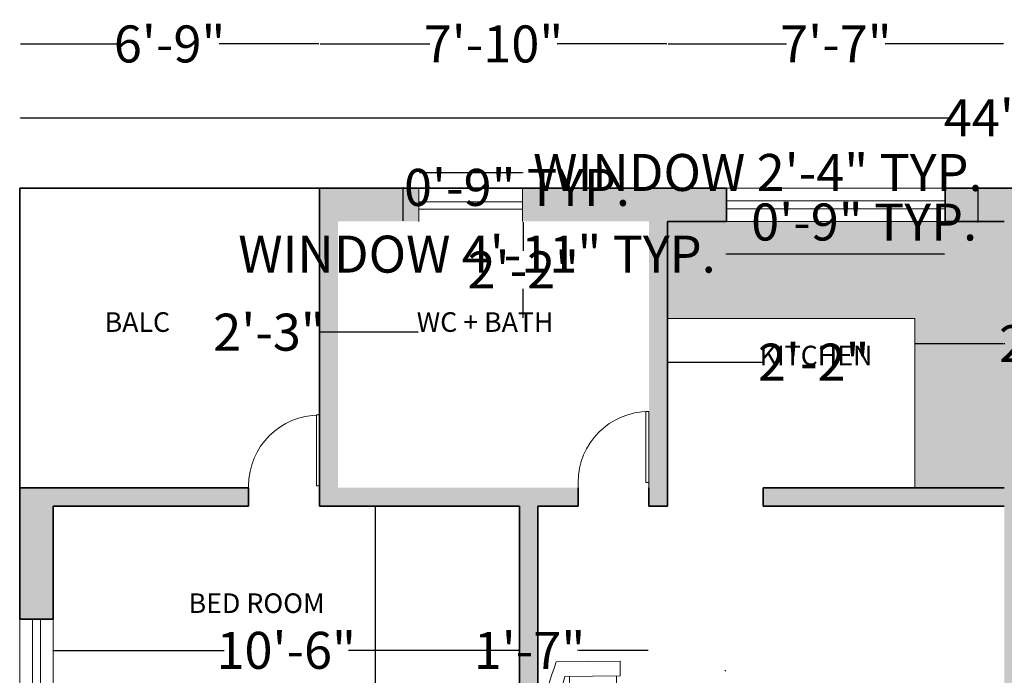
# Model space of a CAD drawing. Units: inches. Extents: x 1198 to 8596, y 144 to 930.
# Tile 4 of 5: x 1348 to 1614, y 753 to 930. Entities that reach past the tile are written whole.
import ezdxf

# ---------------------------------------------------------------- set-up
doc = ezdxf.new("R2010")
doc.units = ezdxf.units.IN
doc.header["$MEASUREMENT"] = 0
doc.layers.get('0').update_dxf_attribs({"color": 50})
for name, color, linetype, lineweight in [('A-ANNO-DIMS', 7, 'Continuous', 18), ('A-AREA-IDEN', 7, 'Continuous', 18), ('A-DOOR', 120, 'Continuous', 18), ('A-FLOR-FIXT', 8, 'Continuous', 18), ('A-FLOR-FIXT-PATT', 150, 'Continuous', 13), ('A-FURN', 11, 'Continuous', 18), ('A-WALL-PATT', 150, 'Continuous', 13), ('WALL', 7, 'Continuous', 35), ('WINDOW', 2, 'Continuous', 18)]:
    doc.layers.add(name, color=color, linetype=linetype, lineweight=lineweight)
doc.styles.get("Standard").update_dxf_attribs({"font": 'arial.ttf'})
doc.dimstyles.get("Standard").update_dxf_attribs({"dimtxt": 10, "dimasz": 0.18, "dimexe": 0.18, "dimexo": 0.0625, "dimgap": 0.09, "dimtad": 0, "dimtih": 1, "dimtoh": 1, "dimdec": 0, "dimzin": 0, "dimdsep": 46, "dimlunit": 3, "dimtxsty": 'Standard', "dimcen": 0.09, "dimse1": 1, "dimse2": 1, "dimadec": 0, "dimazin": 0, "dimtfac": 1, "dimtdec": 0, "dimtofl": 0, "dimtmove": 0, "dimatfit": 3, "dimfxl": 1, "dimtolj": 1, "dimtzin": 0, "dimarcsym": 0})

# ---------------------------------------------------------------- blocks, each defined once
blk = doc.blocks.new('WD_WIN4')
for p, q in [((-0.5, 0.5), (0.5, 0.5)), ((-0.5, 0.12), (0.5, 0.12)), ((-0.5, -0.12), (0.5, -0.12)), ((-0.5, -0.5), (0.5, -0.5))]:
    blk.add_line(p, q)
blk = doc.blocks.new('*U12')
for p, q in [((0, 0), (0, -6)), ((-40, 0), (-40, -6))]:
    blk.add_line(p, q)
blk.add_lwpolyline([(0, 0), (0, 40), (-1.75, 40), (-1.75, 0)], close=True)
blk.add_arc((0, 0), 40, 90, 180)
blk = doc.blocks.new('Sofa - Roundback 7 ft.')
for p, q in [((-12.00002, -32.4421), (-12.00003, -6.5971)), ((11.99997, -32.4421), (11.99998, -6.5971)), ((-36.000027, -34), (-36.000027, -11.4696)), ((35.99998, -34), (35.99998, -11.4696)), ((-35.999844, -13.3819), (35.9998, -13.3819)), ((-36.000027, -32.4421), (35.99998, -32.4421))]:
    blk.add_line(p, q)
for points in [[(-36.000027, -34), (-42.000027, -34), (-42.000027, -8)], [(41.99998, -8), (41.99998, -34), (35.99998, -34)]]:
    blk.add_lwpolyline(points)
for centre, radius, start, end in [((0, -114.25), 114.25, 68.43141, 111.5686), ((-0.00001, -127.1968), 121.1968, 72.72033, 107.2797)]:
    blk.add_arc(centre, radius, start, end)
blk = doc.blocks.new('*D15')
at = {"layer": 'A-ANNO-DIMS', "color": 0, "lineweight": -2, "transparency": 16777216}
for p, q in [((1348.07, 903.88), (1598.92, 903.88)), ((1884.71, 903.88), (1633.85, 903.88))]:
    blk.add_line(p, q, dxfattribs=at)
at = {"layer": 'A-ANNO-DIMS', "color": 0, "transparency": 16777216}
for points in [[(1348.07, 903.91), (1348.07, 903.85), (1347.89, 903.88)], [(1884.71, 903.91), (1884.71, 903.85), (1884.89, 903.88)]]:
    blk.add_solid(points, dxfattribs=at)
at = {"layer": 'Defpoints', "color": 0, "transparency": 16777216}
for p in [(1347.89, 903.88), (1347.89, 884.9), (1884.89, 884.9)]:
    blk.add_point(p, dxfattribs=at)
at = {"layer": 'A-ANNO-DIMS', "color": 0, "transparency": 16777216, "insert": (1616.39, 903.88), "char_height": 10, "attachment_point": 5}
blk.add_mtext('\\A1;44\'-9"', dxfattribs=at)
blk = doc.blocks.new('*D16')
at = {"layer": 'A-ANNO-DIMS', "color": 0, "lineweight": -2, "transparency": 16777216}
for p, q in [((1337.03, 884.72), (1337.03, 736.59)), ((1337.03, 578.08), (1337.03, 726.2))]:
    blk.add_line(p, q, dxfattribs=at)
at = {"layer": 'A-ANNO-DIMS', "color": 0, "transparency": 16777216}
for points in [[(1337, 884.72), (1337.06, 884.72), (1337.03, 884.9)], [(1337, 578.08), (1337.06, 578.08), (1337.03, 577.9)]]:
    blk.add_solid(points, dxfattribs=at)
at = {"layer": 'Defpoints', "color": 0, "transparency": 16777216}
for p in [(1347.89, 884.9), (1337.03, 577.9), (1347.89, 577.9)]:
    blk.add_point(p, dxfattribs=at)
at = {"layer": 'A-ANNO-DIMS', "color": 0, "transparency": 16777216, "insert": (1337.03, 731.4), "char_height": 10, "attachment_point": 5}
blk.add_mtext('\\A1;25\'-7"', dxfattribs=at)
blk = doc.blocks.new('*D17')
at = {"layer": 'A-ANNO-DIMS', "color": 0, "lineweight": -2, "transparency": 16777216}
for p, q in [((1288.75, 884.72), (1288.75, 551.09)), ((1288.75, 207.08), (1288.75, 540.7))]:
    blk.add_line(p, q, dxfattribs=at)
at = {"layer": 'A-ANNO-DIMS', "color": 0, "transparency": 16777216}
for points in [[(1288.72, 884.72), (1288.78, 884.72), (1288.75, 884.9)], [(1288.72, 207.08), (1288.78, 207.08), (1288.75, 206.9)]]:
    blk.add_solid(points, dxfattribs=at)
at = {"layer": 'Defpoints', "color": 0, "transparency": 16777216}
for p in [(1347.89, 884.9), (1288.75, 206.9), (1347.89, 206.9)]:
    blk.add_point(p, dxfattribs=at)
at = {"layer": 'A-ANNO-DIMS', "color": 0, "transparency": 16777216, "insert": (1288.75, 545.9), "char_height": 10, "attachment_point": 5}
blk.add_mtext('\\A1;56\'-6"', dxfattribs=at)
blk = doc.blocks.new('WIN-NARROW-28IN')
for p, q in [((0, 9), (0, 0)), ((28.06, 9), (28.06, 0)), ((0, 5.31), (28.06, 5.31)), ((0, 3.31), (28.06, 3.31))]:
    blk.add_line(p, q)
blk = doc.blocks.new('*D22')
at = {"layer": 'A-ANNO-DIMS', "color": 0, "lineweight": -2, "transparency": 16777216}
for p, q in [((1538.86, 867.04), (1538.68, 867.04)), ((1597.73, 867.04), (1539.04, 867.04))]:
    blk.add_line(p, q, dxfattribs=at)
at = {"layer": 'A-ANNO-DIMS', "color": 0, "transparency": 16777216}
for points in [[(1539.04, 867.07), (1539.04, 867.01), (1538.86, 867.04)], [(1597.73, 867.07), (1597.73, 867.01), (1597.91, 867.04)]]:
    blk.add_solid(points, dxfattribs=at)
at = {"layer": 'Defpoints', "color": 0, "transparency": 16777216}
for p in [(1538.86, 875.9), (1597.91, 875.9), (1538.86, 867.04)]:
    blk.add_point(p, dxfattribs=at)
at = {"layer": 'A-ANNO-DIMS', "color": 0, "transparency": 16777216, "insert": (1471.43, 867.04), "char_height": 10, "attachment_point": 5}
blk.add_mtext('\\A1;WINDOW 4\'-11" TYP.', dxfattribs=at)
blk = doc.blocks.new('*D23')
at = {"layer": 'A-ANNO-DIMS', "color": 0, "lineweight": -2, "transparency": 16777216}
for p, q in [((1606.77, 884.72), (1606.77, 876.08)), ((1606.77, 875.72), (1606.59, 875.72)), ((1606.77, 875.9), (1606.77, 875.72))]:
    blk.add_line(p, q, dxfattribs=at)
at = {"layer": 'A-ANNO-DIMS', "color": 0, "transparency": 16777216}
for points in [[(1606.74, 884.72), (1606.8, 884.72), (1606.77, 884.9)], [(1606.74, 876.08), (1606.8, 876.08), (1606.77, 875.9)]]:
    blk.add_solid(points, dxfattribs=at)
at = {"layer": 'Defpoints', "color": 0, "transparency": 16777216}
for p in [(1597.91, 884.9), (1597.91, 875.9), (1606.77, 875.9)]:
    blk.add_point(p, dxfattribs=at)
at = {"layer": 'A-ANNO-DIMS', "color": 0, "transparency": 16777216, "insert": (1576.02, 875.72), "char_height": 10, "attachment_point": 5}
blk.add_mtext('\\A1;0\'-9" TYP.', dxfattribs=at)
blk = doc.blocks.new('*D24')
at = {"layer": 'A-ANNO-DIMS', "color": 0, "lineweight": -2, "transparency": 16777216}
for p, q in [((1455.87, 889.11), (1483.58, 889.11)), ((1483.76, 889.11), (1483.94, 889.11))]:
    blk.add_line(p, q, dxfattribs=at)
at = {"layer": 'A-ANNO-DIMS', "color": 0, "transparency": 16777216}
for points in [[(1455.87, 889.14), (1455.87, 889.08), (1455.69, 889.11)], [(1483.58, 889.14), (1483.58, 889.08), (1483.76, 889.11)]]:
    blk.add_solid(points, dxfattribs=at)
at = {"layer": 'Defpoints', "color": 0, "transparency": 16777216}
for p in [(1483.76, 889.11), (1455.69, 884.9), (1483.76, 884.9)]:
    blk.add_point(p, dxfattribs=at)
at = {"layer": 'A-ANNO-DIMS', "color": 0, "transparency": 16777216, "insert": (1547.3, 889.11), "char_height": 10, "attachment_point": 5}
blk.add_mtext('\\A1;WINDOW 2\'-4" TYP.', dxfattribs=at)
blk = doc.blocks.new('*D25')
at = {"layer": 'A-ANNO-DIMS', "color": 0, "lineweight": -2, "transparency": 16777216}
for p, q in [((1451.48, 884.9), (1451.48, 885.08)), ((1451.48, 885.08), (1451.66, 885.08)), ((1451.48, 876.08), (1451.48, 884.72))]:
    blk.add_line(p, q, dxfattribs=at)
at = {"layer": 'A-ANNO-DIMS', "color": 0, "transparency": 16777216}
for points in [[(1451.45, 884.72), (1451.51, 884.72), (1451.48, 884.9)], [(1451.45, 876.08), (1451.51, 876.08), (1451.48, 875.9)]]:
    blk.add_solid(points, dxfattribs=at)
at = {"layer": 'Defpoints', "color": 0, "transparency": 16777216}
for p in [(1451.48, 884.9), (1455.69, 884.9), (1455.69, 875.9)]:
    blk.add_point(p, dxfattribs=at)
at = {"layer": 'A-ANNO-DIMS', "color": 0, "transparency": 16777216, "insert": (1482.23, 885.08), "char_height": 10, "attachment_point": 5}
blk.add_mtext('\\A1;0\'-9" TYP.', dxfattribs=at)
blk = doc.blocks.new('*D30')
at = {"layer": 'A-ANNO-DIMS', "color": 0, "lineweight": -2, "transparency": 16777216}
for p, q in [((1348.07, 923.85), (1374.98, 923.85)), ((1428.71, 923.85), (1401.79, 923.85))]:
    blk.add_line(p, q, dxfattribs=at)
at = {"layer": 'A-ANNO-DIMS', "color": 0, "transparency": 16777216}
for points in [[(1348.07, 923.88), (1348.07, 923.82), (1347.89, 923.85)], [(1428.71, 923.88), (1428.71, 923.82), (1428.89, 923.85)]]:
    blk.add_solid(points, dxfattribs=at)
at = {"layer": 'Defpoints', "color": 0, "transparency": 16777216}
for p in [(1428.89, 923.85), (1347.89, 884.9), (1428.89, 884.9)]:
    blk.add_point(p, dxfattribs=at)
at = {"layer": 'A-ANNO-DIMS', "color": 0, "transparency": 16777216, "insert": (1388.39, 923.85), "char_height": 10, "attachment_point": 5}
blk.add_mtext('\\A1;6\'-9"', dxfattribs=at)
blk = doc.blocks.new('*D31')
at = {"layer": 'A-ANNO-DIMS', "color": 0, "lineweight": -2, "transparency": 16777216}
for p, q in [((1429.07, 923.85), (1458.66, 923.85)), ((1522.71, 923.85), (1493.11, 923.85))]:
    blk.add_line(p, q, dxfattribs=at)
at = {"layer": 'A-ANNO-DIMS', "color": 0, "transparency": 16777216}
for points in [[(1429.07, 923.88), (1429.07, 923.82), (1428.89, 923.85)], [(1522.71, 923.88), (1522.71, 923.82), (1522.89, 923.85)]]:
    blk.add_solid(points, dxfattribs=at)
at = {"layer": 'Defpoints', "color": 0, "transparency": 16777216}
for p in [(1522.89, 923.85), (1428.89, 884.9), (1522.89, 875.9)]:
    blk.add_point(p, dxfattribs=at)
at = {"layer": 'A-ANNO-DIMS', "color": 0, "transparency": 16777216, "insert": (1475.89, 923.85), "char_height": 10, "attachment_point": 5}
blk.add_mtext('\\A1;7\'-10"', dxfattribs=at)
blk = doc.blocks.new('*D32')
at = {"layer": 'A-ANNO-DIMS', "color": 0, "lineweight": -2, "transparency": 16777216}
for p, q in [((1523.07, 923.85), (1555.05, 923.85)), ((1613.71, 923.85), (1581.73, 923.85))]:
    blk.add_line(p, q, dxfattribs=at)
at = {"layer": 'A-ANNO-DIMS', "color": 0, "transparency": 16777216}
for points in [[(1523.07, 923.88), (1523.07, 923.82), (1522.89, 923.85)], [(1613.71, 923.88), (1613.71, 923.82), (1613.89, 923.85)]]:
    blk.add_solid(points, dxfattribs=at)
at = {"layer": 'Defpoints', "color": 0, "transparency": 16777216}
for p in [(1613.89, 923.85), (1522.89, 875.9), (1613.89, 875.9)]:
    blk.add_point(p, dxfattribs=at)
at = {"layer": 'A-ANNO-DIMS', "color": 0, "transparency": 16777216, "insert": (1568.39, 923.85), "char_height": 10, "attachment_point": 5}
blk.add_mtext('\\A1;7\'-7"', dxfattribs=at)
blk = doc.blocks.new('*D37')
at = {"layer": 'A-ANNO-DIMS', "color": 0, "lineweight": -2, "transparency": 16777216}
for p, q in [((1357.07, 759.95), (1403.09, 759.95)), ((1482.71, 759.95), (1436.68, 759.95))]:
    blk.add_line(p, q, dxfattribs=at)
at = {"layer": 'A-ANNO-DIMS', "color": 0, "transparency": 16777216}
for points in [[(1357.07, 759.98), (1357.07, 759.92), (1356.89, 759.95)], [(1482.71, 759.98), (1482.71, 759.92), (1482.89, 759.95)]]:
    blk.add_solid(points, dxfattribs=at)
at = {"layer": 'Defpoints', "color": 0, "transparency": 16777216}
for p in [(1356.89, 798.9), (1482.89, 798.9), (1356.89, 759.95)]:
    blk.add_point(p, dxfattribs=at)
at = {"layer": 'A-ANNO-DIMS', "color": 0, "transparency": 16777216, "insert": (1419.89, 759.95), "char_height": 10, "attachment_point": 5}
blk.add_mtext('\\A1;10\'-6"', dxfattribs=at)
blk = doc.blocks.new('*D38')
at = {"layer": 'A-ANNO-DIMS', "color": 0, "lineweight": -2, "transparency": 16777216}
for p, q in [((1443.94, 798.72), (1443.94, 744.09)), ((1443.94, 679.08), (1443.94, 733.7))]:
    blk.add_line(p, q, dxfattribs=at)
at = {"layer": 'A-ANNO-DIMS', "color": 0, "transparency": 16777216}
for points in [[(1443.91, 798.72), (1443.97, 798.72), (1443.94, 798.9)], [(1443.91, 679.08), (1443.97, 679.08), (1443.94, 678.9)]]:
    blk.add_solid(points, dxfattribs=at)
at = {"layer": 'Defpoints', "color": 0, "transparency": 16777216}
for p in [(1443.94, 798.9), (1482.89, 798.9), (1482.89, 678.9)]:
    blk.add_point(p, dxfattribs=at)
at = {"layer": 'A-ANNO-DIMS', "color": 0, "transparency": 16777216, "insert": (1443.94, 738.9), "char_height": 10, "attachment_point": 5}
blk.add_mtext('\\A1;10\'-0"', dxfattribs=at)
blk = doc.blocks.new('*D60')
at = {"layer": 'A-ANNO-DIMS', "color": 0, "lineweight": -2, "transparency": 16777216}
for p, q in [((1483.94, 875.72), (1483.94, 867.89)), ((1483.94, 849.84), (1483.94, 857.67))]:
    blk.add_line(p, q, dxfattribs=at)
at = {"layer": 'A-ANNO-DIMS', "color": 0, "transparency": 16777216}
for points in [[(1483.91, 875.72), (1483.97, 875.72), (1483.94, 875.9)], [(1483.91, 849.84), (1483.97, 849.84), (1483.94, 849.66)]]:
    blk.add_solid(points, dxfattribs=at)
at = {"layer": 'Defpoints', "color": 0, "transparency": 16777216}
for p in [(1483.94, 875.9), (1522.89, 875.9), (1522.89, 849.66)]:
    blk.add_point(p, dxfattribs=at)
at = {"layer": 'A-ANNO-DIMS', "color": 0, "transparency": 16777216, "insert": (1483.94, 862.78), "char_height": 10, "attachment_point": 5}
blk.add_mtext('\\A1;2\'-2"', dxfattribs=at)
blk = doc.blocks.new('*D61')
at = {"layer": 'A-ANNO-DIMS', "color": 0, "lineweight": -2, "transparency": 16777216}
for p, q in [((1589.91, 842.85), (1613.71, 842.85)), ((1613.89, 842.85), (1614.07, 842.85))]:
    blk.add_line(p, q, dxfattribs=at)
at = {"layer": 'A-ANNO-DIMS', "color": 0, "transparency": 16777216}
for points in [[(1589.91, 842.88), (1589.91, 842.82), (1589.73, 842.85)], [(1613.71, 842.88), (1613.71, 842.82), (1613.89, 842.85)]]:
    blk.add_solid(points, dxfattribs=at)
at = {"layer": 'Defpoints', "color": 0, "transparency": 16777216}
for p in [(1613.89, 842.85), (1589.73, 803.9), (1613.89, 803.9)]:
    blk.add_point(p, dxfattribs=at)
at = {"layer": 'A-ANNO-DIMS', "color": 0, "transparency": 16777216, "insert": (1627.53, 842.85), "char_height": 10, "attachment_point": 5}
blk.add_mtext('\\A1;2\'-0"', dxfattribs=at)
blk = doc.blocks.new('*D64')
at = {"layer": 'A-ANNO-DIMS', "color": 0, "lineweight": -2, "transparency": 16777216}
for p, q in [((1523.07, 837.85), (1548.57, 837.85)), ((1548.75, 837.85), (1548.93, 837.85))]:
    blk.add_line(p, q, dxfattribs=at)
at = {"layer": 'A-ANNO-DIMS', "color": 0, "transparency": 16777216}
for points in [[(1523.07, 837.88), (1523.07, 837.82), (1522.89, 837.85)], [(1548.57, 837.88), (1548.57, 837.82), (1548.75, 837.85)]]:
    blk.add_solid(points, dxfattribs=at)
at = {"layer": 'Defpoints', "color": 0, "transparency": 16777216}
for p in [(1548.75, 837.85), (1522.89, 798.9), (1548.75, 798.9)]:
    blk.add_point(p, dxfattribs=at)
at = {"layer": 'A-ANNO-DIMS', "color": 0, "transparency": 16777216, "insert": (1562.4, 837.85), "char_height": 10, "attachment_point": 5}
blk.add_mtext('\\A1;2\'-2"', dxfattribs=at)
blk = doc.blocks.new('*D65')
at = {"layer": 'A-ANNO-DIMS', "color": 0, "lineweight": -2, "transparency": 16777216}
for p, q in [((1498.72, 759.95), (1498.54, 759.95)), ((1517.71, 759.95), (1498.9, 759.95))]:
    blk.add_line(p, q, dxfattribs=at)
at = {"layer": 'A-ANNO-DIMS', "color": 0, "transparency": 16777216}
for points in [[(1498.9, 759.98), (1498.9, 759.92), (1498.72, 759.95)], [(1517.71, 759.98), (1517.71, 759.92), (1517.89, 759.95)]]:
    blk.add_solid(points, dxfattribs=at)
at = {"layer": 'Defpoints', "color": 0, "transparency": 16777216}
for p in [(1498.72, 798.9), (1517.89, 798.9), (1498.72, 759.95)]:
    blk.add_point(p, dxfattribs=at)
at = {"layer": 'A-ANNO-DIMS', "color": 0, "transparency": 16777216, "insert": (1485.62, 759.95), "char_height": 10, "attachment_point": 5}
blk.add_mtext('\\A1;1\'-7"', dxfattribs=at)
blk = doc.blocks.new('*D66')
at = {"layer": 'A-ANNO-DIMS', "color": 0, "lineweight": -2, "transparency": 16777216}
for p, q in [((1428.89, 845.95), (1428.71, 845.95)), ((1455.51, 845.95), (1429.07, 845.95))]:
    blk.add_line(p, q, dxfattribs=at)
at = {"layer": 'A-ANNO-DIMS', "color": 0, "transparency": 16777216}
for points in [[(1429.07, 845.98), (1429.07, 845.92), (1428.89, 845.95)], [(1455.51, 845.98), (1455.51, 845.92), (1455.69, 845.95)]]:
    blk.add_solid(points, dxfattribs=at)
at = {"layer": 'Defpoints', "color": 0, "transparency": 16777216}
for p in [(1428.89, 884.9), (1455.69, 884.9), (1428.89, 845.95)]:
    blk.add_point(p, dxfattribs=at)
at = {"layer": 'A-ANNO-DIMS', "color": 0, "transparency": 16777216, "insert": (1415.24, 845.95), "char_height": 10, "attachment_point": 5}
blk.add_mtext('\\A1;2\'-3"', dxfattribs=at)
blk = doc.blocks.new('*D69')
at = {"layer": 'A-ANNO-DIMS', "color": 0, "lineweight": -2, "transparency": 16777216}
for p, q in [((1538.43, 754.55), (1538.61, 754.55)), ((1538.52, 754.46), (1538.52, 754.64)), ((1538.53, 633.54), (1538.53, 678.74)), ((1538.71, 633.54), (1538.53, 633.54))]:
    blk.add_line(p, q, dxfattribs=at)
at = {"layer": 'A-ANNO-DIMS', "color": 0, "transparency": 16777216}
blk.add_solid([(1538.56, 678.74), (1538.5, 678.74), (1538.53, 678.92)], dxfattribs=at)
at = {"layer": 'Defpoints', "color": 0, "transparency": 16777216}
for p in [(1538.52, 754.55), (1538.53, 678.92)]:
    blk.add_point(p, dxfattribs=at)
at = {"layer": 'A-ANNO-DIMS', "color": 0, "transparency": 16777216, "insert": (1579.29, 633.54), "char_height": 10, "attachment_point": 5}
blk.add_mtext('\\A1;6X R6\'-3 1/2"', dxfattribs=at)

msp = doc.modelspace()

# ---------------------------------------------------------------- hatches: boundary and pattern name
at = {"layer": 'A-FLOR-FIXT-PATT', "transparency": 33554607}
h = msp.add_hatch(dxfattribs=at)
h.set_pattern_fill('ACAD_ISO04W100', color=256, scale=0.1)
h.set_pattern_definition([(0, (0, 0), (0, 0.5), [2.4, -0.3, 0.05, -0.3])])
h.paths.add_polyline_path([(1613.89, 875.9), (1597.91, 875.9), (1538.86, 875.9), (1522.89, 875.9), (1522.89, 849.66), (1589.73, 849.66), (1589.73, 803.9), (1613.89, 803.9)])
h.paths.add_polyline_path([(1709.89, 875.9), (1693.91, 875.9), (1634.86, 875.9), (1618.89, 875.9), (1618.89, 803.9), (1645.58, 803.9), (1645.58, 852.52), (1709.89, 852.52)])
at = {"layer": 'A-WALL-PATT'}
h = msp.add_hatch(color=256, dxfattribs=at)
h.dxf.hatch_style = 1
h.paths.add_polyline_path([(1884.89, 495.9), (1884.89, 534.37), (1875.89, 534.37), (1875.89, 500.9), (1823.11, 500.9), (1823.11, 495.9)])
h.paths.add_polyline_path([(1875.89, 593.42), (1884.89, 593.42), (1884.89, 685.87), (1875.89, 685.87), (1875.89, 631.9), (1749.89, 631.9), (1749.89, 766.08), (1744.89, 766.08), (1744.89, 631.97), (1618.79, 631.97), (1613.89, 631.97), (1613.89, 593.42), (1622.89, 593.42), (1622.89, 626.9), (1744.89, 626.9), (1744.89, 537.33), (1749.89, 537.33), (1749.89, 626.9), (1875.89, 626.9)])
h.paths.add_polyline_path([(1884.89, 206.9), (1884.89, 249.37), (1875.89, 249.37), (1875.89, 215.9), (1842.41, 215.9), (1842.41, 206.9)])
h.paths.add_polyline_path([(1783.36, 206.9), (1783.36, 215.9), (1749.89, 215.9), (1749.89, 308.42), (1744.89, 308.42), (1744.89, 215.9), (1713.41, 215.9), (1713.41, 206.9)])
h.paths.add_polyline_path([(1654.36, 206.9), (1654.36, 215.9), (1622.89, 215.9), (1622.89, 249.37), (1613.89, 249.37), (1613.89, 206.9)])
h.paths.add_polyline_path([(1613.89, 334.34), (1622.89, 334.34), (1622.89, 341.9), (1622.89, 368.41), (1613.89, 368.41)])
h.paths.add_polyline_path([(1613.89, 396.47), (1622.89, 396.47), (1622.89, 418.9), (1710.09, 418.9), (1710.09, 400.51), (1709.89, 346.77), (1709.89, 341.9), (1714.89, 341.9), (1714.89, 346.9), (1714.88, 366), (1714.89, 418.9), (1798.89, 418.9), (1798.89, 346.9), (1734.06, 346.9), (1734.07, 343.96), (1734.06, 341.9), (1744.89, 341.9), (1744.89, 334.34), (1749.89, 334.34), (1749.89, 341.9), (1803.93, 341.9), (1803.93, 346.9), (1803.89, 346.9), (1803.89, 418.9), (1884.89, 418.9), (1884.89, 423.9), (1803.89, 423.9), (1803.89, 495.9), (1803.93, 500.9), (1749.89, 500.9), (1749.89, 511.41), (1747.24, 511.41), (1744.89, 511.41), (1744.89, 500.9), (1734.06, 500.9), (1734.06, 495.9), (1798.89, 495.9), (1798.89, 423.9), (1714.89, 423.9), (1714.89, 495.9), (1714.89, 500.9), (1709.89, 500.9), (1709.89, 496.89), (1709.89, 495.9), (1709.89, 423.9), (1622.89, 423.9), (1622.89, 446.07), (1613.89, 446.07)])
h.paths.add_polyline_path([(1613.89, 474.13), (1622.89, 474.13), (1622.89, 495.9), (1645.93, 495.9), (1683.97, 495.9), (1683.89, 500.9), (1648.32, 500.9), (1648.32, 500.88), (1622.41, 500.86), (1618.52, 500.86), (1613.89, 500.9)])
h.paths.add_polyline_path([(1613.89, 526.77), (1613.89, 534.37), (1622.89, 534.37), (1622.89, 526.77, -0.395914), (1648.3, 502.01), (1648.32, 502.01), (1648.32, 500.88), (1622.41, 500.86), (1622.41, 502), (1648.3, 502.01, 0.395914), (1622.89, 526.77)])
h.paths.add_polyline_path([(1875.89, 744.92), (1884.89, 744.92), (1884.89, 803.9), (1823.06, 803.9), (1823.06, 798.9), (1875.89, 798.9)])
h.paths.add_polyline_path([(1798.89, 803.9), (1734.06, 803.9), (1734.06, 802.45), (1734.06, 798.9), (1744.89, 798.9), (1744.89, 792), (1749.89, 792), (1749.89, 798.9), (1803.89, 798.9), (1803.89, 803.9), (1803.89, 884.9), (1774.16, 884.9), (1774.16, 875.9), (1798.89, 875.9)])
h.paths.add_polyline_path([(1746.09, 875.9), (1746.09, 884.9), (1693.91, 884.9), (1693.91, 875.9), (1709.89, 875.9), (1709.89, 803.9), (1709.89, 798.9), (1714.89, 798.9), (1714.89, 803.9), (1714.89, 875.9)])
h.paths.add_polyline_path([(1618.89, 798.9), (1683.96, 798.9), (1683.96, 803.9), (1618.89, 803.9), (1618.89, 875.9), (1634.86, 875.9), (1634.86, 884.9), (1597.91, 884.9), (1597.91, 875.9), (1613.89, 875.9), (1613.89, 803.9), (1548.75, 803.9), (1548.75, 798.9), (1613.89, 798.9), (1613.89, 657.88), (1618.8, 657.88)])
h.paths.add_polyline_path([(1522.89, 875.9), (1538.86, 875.9), (1538.86, 884.9), (1483.76, 884.9), (1483.76, 875.9), (1517.89, 875.9), (1517.89, 803.9), (1517.89, 802.46), (1517.89, 798.9), (1522.89, 798.9), (1522.89, 803.9)], flags=17)
h.paths.add_polyline_path([(1428.89, 884.9), (1428.89, 803.9), (1428.89, 798.9), (1482.89, 798.9), (1482.89, 678.9), (1356.89, 678.9), (1356.89, 709.37), (1347.89, 709.37), (1347.89, 577.9), (1508.89, 577.9), (1508.89, 586.9), (1356.89, 586.9), (1356.89, 673.9), (1565.89, 673.9), (1565.89, 678.9), (1487.89, 678.9), (1487.89, 798.9), (1498.72, 798.9), (1498.72, 803.9), (1433.89, 803.9), (1433.89, 875.9), (1455.69, 875.9), (1455.69, 884.9)])
h.paths.add_polyline_path([(1356.89, 798.9), (1409.72, 798.9), (1409.72, 803.9), (1347.89, 803.9), (1347.89, 768.42), (1356.89, 768.42)], flags=17)
h.paths.add_polyline_path([(1884.89, 346.9), (1823.09, 346.9, -0.008805), (1823.1, 346.22), (1823.11, 343.35), (1823.09, 341.9), (1875.89, 341.9), (1875.89, 308.42), (1884.89, 308.42)])

# ---------------------------------------------------------------- linework, layer by layer
at = {"layer": 'A-FLOR-FIXT'}
for p, q in [((1589.73, 849.66), (1522.89, 849.66)), ((1589.73, 803.9), (1589.73, 849.66))]:
    msp.add_line(p, q, dxfattribs=at)
at = {"layer": 'WALL'}
for p, q in [((1347.89, 884.9), (1538.86, 884.9)), ((1347.89, 768.42), (1347.89, 884.9)), ((1428.89, 803.9), (1428.89, 884.9)), ((1538.86, 875.9), (1538.86, 884.9)), ((1597.91, 884.9), (1634.86, 884.9)), ((1597.91, 875.9), (1597.91, 884.9)), ((1522.89, 803.9), (1522.89, 875.9)), ((1522.89, 875.9), (1538.86, 875.9)), ((1597.91, 875.9), (1613.89, 875.9)), ((1347.89, 803.9), (1409.72, 803.9)), ((1409.72, 803.9), (1409.72, 798.9)), ((1428.89, 803.9), (1428.89, 798.9)), ((1498.72, 803.89), (1498.72, 798.9)), ((1517.89, 803.9), (1517.89, 798.9)), ((1522.89, 803.9), (1522.89, 798.9)), ((1548.75, 803.9), (1613.89, 803.9)), ((1548.75, 803.9), (1548.75, 798.9)), ((1356.89, 798.9), (1409.72, 798.9)), ((1356.89, 768.42), (1356.89, 798.9)), ((1428.89, 798.9), (1482.89, 798.9)), ((1482.89, 678.9), (1482.89, 798.9)), ((1487.89, 678.9), (1487.89, 798.9)), ((1487.89, 798.9), (1498.72, 798.9)), ((1517.89, 798.9), (1522.89, 798.9)), ((1548.75, 798.9), (1613.89, 798.9)), ((1356.89, 768.42), (1347.89, 768.42))]:
    msp.add_line(p, q, dxfattribs=at)

# ---------------------------------------------------------------- block references
at = {"layer": 'A-DOOR', "xscale": 0.4792807635590344, "yscale": 0.4792807635590344, "zscale": 0.4792807635590344, "rotation": 0.0341043339832885}
for p in [(1428.89, 804.4), (1517.89, 805.33)]:
    msp.add_blockref('*U12', p, dxfattribs=at)
at = {"layer": 'A-FURN', "xscale": 0.6619781710857556, "yscale": 0.6619781710857556, "zscale": 0.6619781710857556, "rotation": 90.68030024111884}
msp.add_blockref('Sofa - Roundback 7 ft.', (1487.89, 728.94), dxfattribs=at)
at = {"layer": 'WINDOW'}
msp.add_blockref('WIN-NARROW-28IN', (1455.69, 875.9), dxfattribs=at)
at = {"layer": 'WINDOW', "xscale": 59.05511811023622, "zscale": 59.05511811023622}
for p, yscale, rotation in [((1568.39, 880.4), 9.000000000000568, 180.0000000000002), ((1352.39, 738.9), 9.000000000000227, 89.99999999999957)]:
    msp.add_blockref('WD_WIN4', p, dxfattribs=dict(at, yscale=yscale, rotation=rotation))

# ---------------------------------------------------------------- texts
at = {"layer": 'A-AREA-IDEN'}
for s, p in [('BALC', (1370.83, 846.03)), ('WC + BATH', (1455.14, 846.03)), (' KITCHEN', (1546.14, 836.99)), (' BED ROOM', (1391.9, 770.05))]:
    msp.add_text(s, height=5.299, dxfattribs=at).set_placement(p)

# ---------------------------------------------------------------- dimensions: what is measured, and where the dimension line sits
at = {"layer": 'A-ANNO-DIMS'}
for base, p1, p2, override, picture, middle in [((1428.89, 923.85), (1347.89, 884.9), (1428.89, 884.9), {"dimdec": 1, "dimlfac": 1, "dimrnd": 0, "dimzin": 1, "dimdsep": 46, "dimlunit": 4, "dimfrac": 2}, '*D30', (1388.39, 923.85)), ((1522.89, 923.85), (1428.89, 884.9), (1522.89, 875.9), {"dimdec": 1, "dimlfac": 1, "dimrnd": 0, "dimzin": 1, "dimdsep": 46, "dimlunit": 4, "dimfrac": 2}, '*D31', (1475.89, 923.85)), ((1613.89, 923.85), (1522.89, 875.9), (1613.89, 875.9), {"dimdec": 1, "dimlfac": 1, "dimrnd": 0, "dimzin": 1, "dimdsep": 46, "dimlunit": 4, "dimfrac": 2}, '*D32', (1568.39, 923.85)), ((1347.89, 903.88), (1884.89, 884.9), (1347.89, 884.9), {"dimclrd": 0, "dimclre": 0, "dimclrt": 0}, '*D15', (1616.39, 903.88))]:
    dim = msp.add_linear_dim(base=base, p1=p1, p2=p2, dimstyle='Standard', override=override, dxfattribs=at)
    dim.commit()
    dim.dimension.update_dxf_attribs({"geometry": picture, "text_midpoint": middle})
dim = msp.add_linear_dim(base=(1483.76, 889.11), p1=(1455.69, 884.9), p2=(1483.76, 884.9), text='WINDOW <> TYP.', dimstyle='Standard', override={"dimdec": 1, "dimlfac": 1, "dimrnd": 0, "dimzin": 1, "dimdsep": 46, "dimlunit": 4, "dimfrac": 2}, dxfattribs=at)
dim.commit()
dim.dimension.update_dxf_attribs({"geometry": '*D24', "text_midpoint": (1547.3, 889.11)})
for base, p1, p2, angle, text, picture, middle in [((1451.48, 884.9), (1455.69, 875.9), (1455.69, 884.9), 90, '<> TYP.', '*D25', (1482.23, 885.08)), ((1538.8587, 867.0383), (1597.9138, 875.8966), (1538.8587, 875.8966), 180, 'WINDOW <> TYP.', '*D22', (1471.4332, 867.0383)), ((1606.77, 875.9), (1597.91, 884.9), (1597.91, 875.9), 270, '<> TYP.', '*D23', (1576.02, 875.72))]:
    dim = msp.add_linear_dim(base=base, p1=p1, p2=p2, angle=angle, text=text, dimstyle='Standard', override={"dimdec": 1, "dimlfac": 1, "dimrnd": 0, "dimzin": 1, "dimdsep": 46, "dimlunit": 4, "dimfrac": 2}, dxfattribs=at)
    dim.commit()
    dim.dimension.update_dxf_attribs({"geometry": picture, "text_midpoint": middle})
for base, p1, p2, angle, override, picture, middle in [((1288.75, 206.9), (1347.89, 884.9), (1347.89, 206.9), 90, {"dimclrd": 0, "dimclre": 0, "dimclrt": 0}, '*D17', (1288.75, 545.9)), ((1337.03, 577.9), (1347.89, 884.9), (1347.89, 577.9), 90, {"dimclrd": 0, "dimclre": 0, "dimclrt": 0}, '*D16', (1337.03, 731.4)), ((1428.89, 845.95), (1455.69, 884.9), (1428.89, 884.9), 180, {"dimdec": 1, "dimlfac": 1, "dimrnd": 0, "dimzin": 1, "dimdsep": 46, "dimlunit": 4, "dimfrac": 2}, '*D66', (1415.24, 845.95)), ((1483.94, 875.9), (1522.89, 849.66), (1522.89, 875.9), 90, {"dimdec": 1, "dimlfac": 1, "dimrnd": 0, "dimzin": 1, "dimdsep": 46, "dimlunit": 4, "dimfrac": 2}, '*D60', (1483.94, 862.78)), ((1613.89, 842.85), (1589.73, 803.9), (1613.89, 803.9), 0, {"dimdec": 1, "dimlfac": 1, "dimrnd": 0, "dimzin": 1, "dimdsep": 46, "dimlunit": 4, "dimfrac": 2}, '*D61', (1627.53, 842.85)), ((1548.75, 837.85), (1522.89, 798.9), (1548.75, 798.9), 0, {"dimdec": 1, "dimlfac": 1, "dimrnd": 0, "dimzin": 1, "dimdsep": 46, "dimlunit": 4, "dimfrac": 2}, '*D64', (1562.4, 837.85)), ((1356.89, 759.95), (1482.89, 798.9), (1356.89, 798.9), 180, {"dimdec": 1, "dimlfac": 1, "dimrnd": 0, "dimzin": 1, "dimdsep": 46, "dimlunit": 4, "dimfrac": 2}, '*D37', (1419.89, 759.95)), ((1443.94, 798.9), (1482.89, 678.9), (1482.89, 798.9), 90, {"dimdec": 1, "dimlfac": 1, "dimrnd": 0, "dimzin": 1, "dimdsep": 46, "dimlunit": 4, "dimfrac": 2}, '*D38', (1443.94, 738.9)), ((1498.72, 759.95), (1517.89, 798.9), (1498.72, 798.9), 180, {"dimdec": 1, "dimlfac": 1, "dimrnd": 0, "dimzin": 1, "dimdsep": 46, "dimlunit": 4, "dimfrac": 2}, '*D65', (1485.62, 759.95))]:
    dim = msp.add_linear_dim(base=base, p1=p1, p2=p2, angle=angle, dimstyle='Standard', override=override, dxfattribs=at)
    dim.commit()
    dim.dimension.update_dxf_attribs({"geometry": picture, "text_midpoint": middle})
dim = msp.add_radius_dim(center=(1538.52, 754.55), mpoint=(1538.53, 678.92), text='6X <>', dimstyle='Standard', override={"dimdec": 1, "dimlfac": 1, "dimrnd": 0, "dimzin": 1, "dimdsep": 46, "dimlunit": 4, "dimfrac": 2}, dxfattribs=at)
dim.commit()
dim.dimension.update_dxf_attribs({"geometry": '*D69', "text_midpoint": (1579.29, 633.54), "dimtype": 164})

doc.saveas('drawing.dxf')
